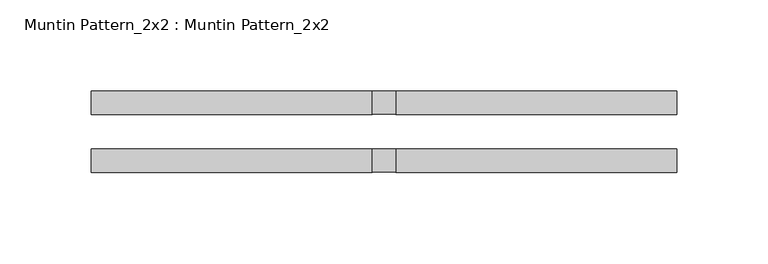
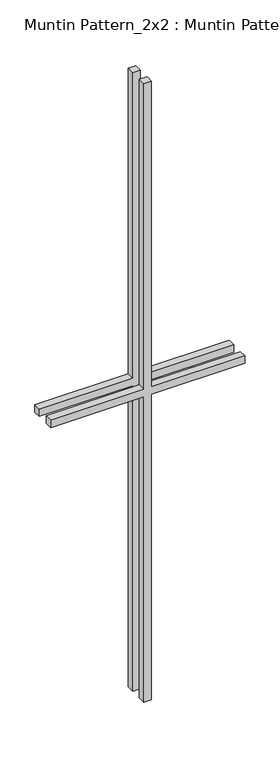
"""IFC4 building model written with IfcOpenShell, lengths in millimetres: proxy geometry, Muntin Pattern_2x2 : Muntin Pattern_2x2."""

from ifc_helpers import new_model, si_unit, frame, origin, place, context, project, spatial, polyline, outline, extrude, source, transform, mapped, element, save


def muntin_pattern_2x2_muntin_pattern_2x2_1acec82f(model_context):
    return source(origin(), model_context, "Body", "SweptSolid", [
        extrude(outline(polyline([(546.1, -6.35), (546.1, -160.3375), (533.4, -160.3375), (533.4, -6.35), (0.0, -6.35), (0.0, 6.35), (533.4, 6.35), (533.4, 160.3375), (546.1, 160.3375), (546.1, 6.35), (1079.5, 6.35), (1079.5, -6.35), (546.1, -6.35)])), frame((0.0, 9.525, 0.0), z_axis=(0.0, 1.0, 0.0), x_axis=(0.0, 0.0, 1.0)), (0.0, 0.0, 1.0), 12.7),
        extrude(outline(polyline([(546.1, -6.35), (546.1, -160.3375), (533.4, -160.3375), (533.4, -6.35), (0.0, -6.35), (0.0, 6.35), (533.4, 6.35), (533.4, 160.3375), (546.1, 160.3375), (546.1, 6.35), (1079.5, 6.35), (1079.5, -6.35), (546.1, -6.35)])), frame((0.0, -22.225, 0.0), z_axis=(0.0, 1.0, 0.0), x_axis=(0.0, 0.0, 1.0)), (0.0, 0.0, 1.0), 12.7),
    ])


if __name__ == "__main__":
    model = new_model("IFC4")
    model_context = context("Model", 3, world=origin())
    ifc_project = project(units=[si_unit("LENGTHUNIT", "METRE", prefix="MILLI")], contexts=[model_context])
    site = spatial("IfcSite", under=ifc_project)
    building = spatial("IfcBuilding", under=site)
    placement = place(None, origin())
    muntin_pattern_2x2_muntin_pattern_2x2_shape = muntin_pattern_2x2_muntin_pattern_2x2_1acec82f(model_context)
    element("IfcBuildingElementProxy", 1, Name="Muntin Pattern_2x2 : Muntin Pattern_2x2", ObjectType="Muntin Pattern_2x2 : Muntin Pattern_2x2", at=placement, inside=building, context=model_context, shape_type="MappedRepresentation", body=[
        mapped(muntin_pattern_2x2_muntin_pattern_2x2_shape, transform((0.0, 0.0, 0.0), x_axis=(1.0, 0.0, 0.0), y_axis=(0.0, 1.0, 0.0), z_axis=(0.0, 0.0, 1.0))),
    ])
    save(model, "model.ifc")

# Revit data of these elements
# Type "Muntin Pattern_2x2 : Muntin Pattern_2x2"
#   Width [instance default] = 4' - 0"
#   Thickness = 0' - 0 1/2"
#   Height [instance default] = 4' - 0"
#   Distance = 0' - 0 3/4"
#   Interior Material [instance default] = none
#   Exterior Material [instance default] = none
#   Default Elevation = 0
# Element 1 (IfcBuildingElementProxy, "Muntin Pattern_2x2 : Muntin Pattern_2x2")
#   Width = 1' - 0 5/8"
#   Height = 3' - 6 1/2"
#   Interior Material = Wood - Stained
#   Exterior Material = Clad - White
#   Materials on its faces: "Clad - White", "Wood - Stained"
# Materials
#   "Clad - White": class "Wood", colour RGB 242 242 238, transparency 0, Cost = 0
#   "Wood - Stained": class "Wood", colour RGB 224 178 126, transparency 0, Cost = 0
